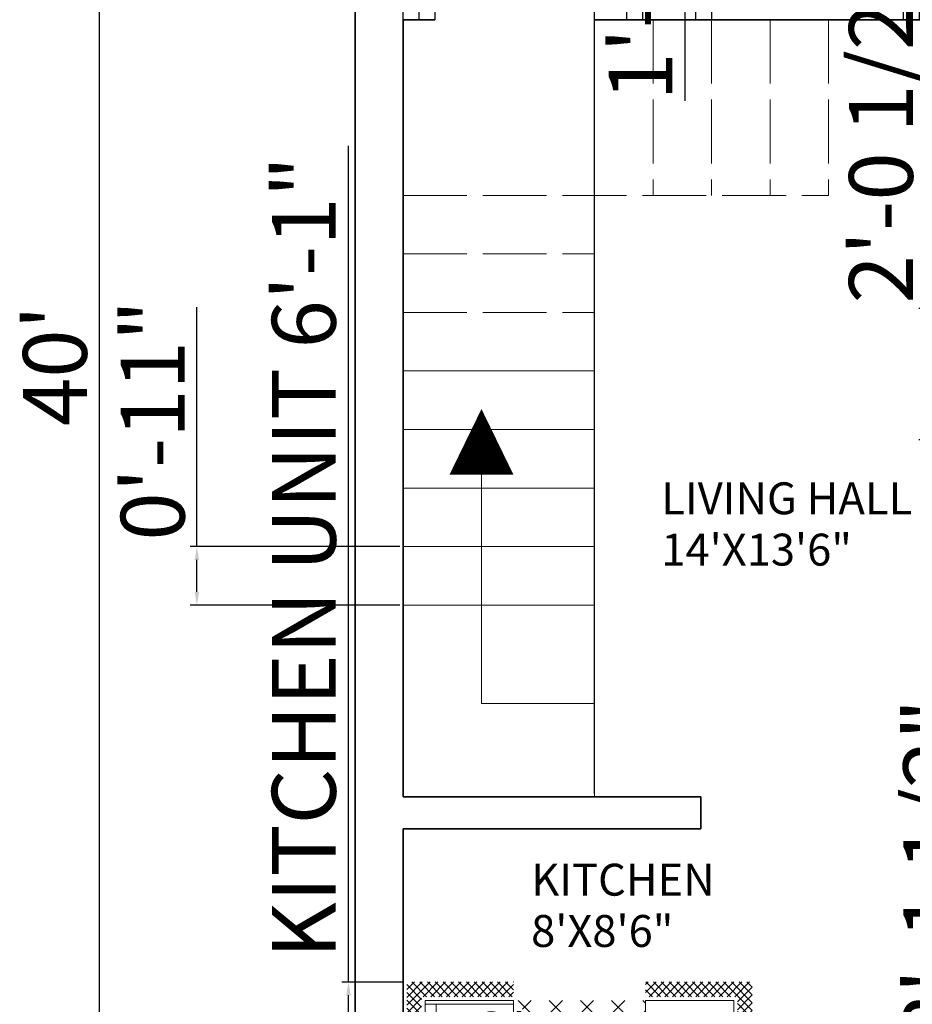
# Model space of a CAD drawing. Units: inches. Extents: x 2353 to 2961, y 642 to 1248.
# Tile 2 of 5: x 2353 to 2520, y 840 to 1025. Entities that reach past the tile are written whole.
import ezdxf

# ---------------------------------------------------------------- set-up
doc = ezdxf.new("R2010")
doc.units = ezdxf.units.IN
doc.linetypes.add('ACAD_ISO02W100', pattern=[15, 12, -3])
for name, color, linetype, lineweight in [('A-ANNO-DIMS', 2, 'Continuous', 18), ('A-AREA-IDEN', 7, 'Continuous', 18), ('A-DOOR', 4, 'Continuous', 25), ('A-FLOR-FIXT', 9, 'Continuous', 18), ('A-FLOR-STRS', 7, 'Continuous', 18), ('A-FLOR-STRS-OVHD', 7, 'ACAD_ISO02W100', 18), ('A-WALL', 7, 'Continuous', 35)]:
    doc.layers.add(name, color=color, linetype=linetype, lineweight=lineweight)
doc.styles.get("Standard").update_dxf_attribs({"font": 'arial.ttf'})
doc.dimstyles.new('ISO-25', dxfattribs={"dimtxt": 12, "dimasz": 2.5, "dimexe": 1.25, "dimexo": 0.625, "dimtad": 1, "dimdec": 1, "dimlunit": 3, "dimtxsty": 'Standard', "dimcen": 2.5, "dimadec": 0, "dimazin": 0, "dimtfac": 1, "dimtdec": 1, "dimtmove": 0, "dimatfit": 3, "dimfxl": 1, "dimarcsym": 0})

# ---------------------------------------------------------------- blocks, each defined once
blk = doc.blocks.new('Kitchen Layout - 7 x 8 ft')
for p, q in [((-5, 81.32), (2.68, 89)), ((-5, 83.44), (0.56, 89)), ((-5, 85.56), (-1.56, 89)), ((-5, 87.68), (-3.68, 89)), ((-1, 84.97), (-5, 88.97)), ((1.09, 85), (-2.91, 89)), ((3.21, 85), (-0.79, 89)), ((0.81, 85), (4.81, 89)), ((5.34, 85), (1.34, 89)), ((2.93, 85), (6.93, 89)), ((7.46, 85), (3.46, 89)), ((5.05, 85), (9.05, 89)), ((9.58, 85), (5.58, 89)), ((7.17, 85), (11.17, 89)), ((11.7, 85), (7.7, 89)), ((9.29, 85), (13.29, 89)), ((13.82, 85), (9.82, 89)), ((11.41, 85), (15.41, 89)), ((15.94, 85), (11.94, 89)), ((13.53, 85), (17.53, 89)), ((18.06, 85), (14.06, 89)), ((15.65, 85), (19.65, 89)), ((20.18, 85), (16.18, 89)), ((17.78, 85), (21.78, 89)), ((22.31, 85), (18.31, 89)), ((19.9, 85), (23.9, 89)), ((24.43, 85), (20.43, 89)), ((22.02, 85), (26.02, 89)), ((26.55, 85), (22.55, 89)), ((24.14, 85), (28.14, 89)), ((28.67, 85), (24.67, 89)), ((26.26, 85), (30.26, 89)), ((30.79, 85), (26.79, 89)), ((28.38, 85), (32.38, 89)), ((32.91, 85), (28.91, 89)), ((30.5, 85), (34.5, 89)), ((35.03, 85), (31.03, 89)), ((32.63, 85), (36.63, 89)), ((37.16, 85), (33.16, 89)), ((34.75, 85), (38.75, 89)), ((39.28, 85), (35.28, 89)), ((36.87, 85), (40.87, 89)), ((41.4, 85), (37.4, 89)), ((38.99, 85), (42.99, 89)), ((43.52, 85), (39.52, 89)), ((41.11, 85), (45.11, 89)), ((45.64, 85), (41.64, 89)), ((43.23, 85), (47.23, 89)), ((47.76, 85), (43.76, 89)), ((45.35, 85), (49.35, 89)), ((49.88, 85), (45.88, 89)), ((47.47, 85), (51.47, 89)), ((52, 85), (48, 89)), ((49.6, 85), (53.6, 89)), ((54.13, 85), (50.13, 89)), ((51.72, 85), (55.72, 89)), ((56.25, 85), (52.25, 89)), ((53.84, 85), (57.84, 89)), ((58.37, 85), (54.37, 89)), ((55.96, 85), (59.96, 89)), ((60.49, 85), (56.49, 89)), ((58.08, 85), (62.08, 89)), ((62.61, 85), (58.61, 89)), ((60.2, 85), (64.2, 89)), ((64.73, 85), (60.73, 89)), ((62.32, 85), (66.32, 89)), ((66.85, 85), (62.85, 89)), ((64.45, 85), (68.45, 89)), ((68.97, 85), (64.97, 89)), ((66.57, 85), (70.57, 89)), ((71.1, 85), (67.1, 89)), ((68.69, 85), (72.69, 89)), ((73.22, 85), (69.22, 89)), ((70.81, 85), (74.81, 89)), ((75.34, 85), (71.34, 89)), ((72.93, 85), (76.93, 89)), ((77.46, 85), (73.46, 89)), ((75.05, 85), (79.05, 89)), ((79.58, 85), (75.58, 89)), ((77.17, 85), (81.17, 89)), ((81.7, 85), (77.7, 89)), ((79.29, 85), (83.29, 89)), ((83.82, 85), (79.82, 89)), ((81.42, 85), (85.42, 89)), ((85.95, 85), (81.95, 89)), ((83.54, 85), (87.54, 89)), ((88.07, 85), (84.07, 89)), ((85.66, 85), (89.66, 89)), ((90.19, 85), (86.19, 89)), ((87.78, 85), (91.78, 89)), ((92.31, 85), (88.31, 89)), ((89.9, 85), (93.9, 89)), ((94.43, 85), (90.43, 89)), ((92.02, 85), (96.02, 89)), ((96.55, 85), (92.55, 89)), ((94.14, 85), (98.14, 89)), ((101, 82.67), (94.67, 89)), ((96.27, 85), (100.27, 89)), ((101, 84.79), (96.79, 89)), ((101, 86.92), (98.92, 89)), ((-1, 82.85), (-5, 86.85)), ((97, 83.61), (101, 87.61)), ((-1, 80.73), (-5, 84.73)), ((-5, 79.19), (-1, 83.19)), ((34, 84), (96, 84)), ((34, 60), (34, 84)), ((96, 84), (96, 60)), ((97, 81.49), (101, 85.49)), ((101, 80.55), (97, 84.55)), ((97, 79.37), (101, 83.37)), ((-1, 78.61), (-5, 82.61)), ((-5, 77.07), (-1, 81.07)), ((-1, 76.49), (-5, 80.49)), ((74, 81), (95, 81)), ((101, 78.43), (97, 82.43)), ((97, 77.25), (101, 81.25)), ((-5, 74.95), (-1, 78.95)), ((-1, 74.36), (-5, 78.36)), ((101, 76.31), (97, 80.31)), ((97, 75.13), (101, 79.13)), ((101, 74.19), (97, 78.19)), ((-5, 72.83), (-1, 76.83)), ((-1, 72.24), (-5, 76.24)), ((97, 73.01), (101, 77.01)), ((101, 72.07), (97, 76.07)), ((-5, 70.71), (-1, 74.71)), ((-1, 70.12), (-5, 74.12)), ((-5, 68.59), (-1, 72.59)), ((97, 70.89), (101, 74.89)), ((101, 69.95), (97, 73.95)), ((97, 68.76), (101, 72.76)), ((-1, 68), (-5, 72)), ((-5, 66.47), (-1, 70.47)), ((-1, 65.88), (-5, 69.88)), ((101, 67.82), (97, 71.82)), ((97, 66.64), (101, 70.64)), ((101, 65.7), (97, 69.7)), ((-5, 64.35), (-1, 68.35)), ((-1, 63.76), (-5, 67.76)), ((97, 64.52), (101, 68.52)), ((101, 63.58), (97, 67.58)), ((-5, 62.22), (-1, 66.22)), ((-1, 61.64), (-5, 65.64)), ((97, 62.4), (101, 66.4)), ((101, 61.46), (97, 65.46)), ((-5, 60.1), (-1, 64.1)), ((-1, 59.52), (-5, 63.52)), ((-5, 57.98), (-1, 61.98)), ((97, 60.28), (101, 64.28)), ((100.34, 60), (97, 63.34)), ((98.84, 60), (101, 62.16)), ((-1, 57.39), (-5, 61.39)), ((-1.73, 56), (-5, 59.27)), ((-4.86, 56), (-1, 59.86)), ((10.4, 24), (45.9, 59.5)), ((18.88, 24), (54.38, 59.5)), ((27.37, 24), (62.87, 59.5)), ((33.03, 55.11), (37.41, 59.5)), ((96, 60), (34, 60)), ((35.85, 24), (71.35, 59.5)), ((76.2, 24), (40.7, 59.5)), ((84.68, 24), (49.18, 59.5)), ((93.17, 24), (57.67, 59.5)), ((96, 29.65), (66.15, 59.5)), ((80, 60), (80, 59)), ((82, 59), (82, 60)), ((87, 59), (87, 60)), ((89, 60), (89, 59)), ((98.22, 60), (97, 61.22)), ((100.96, 60), (101, 60.04)), ((-3.85, 56), (-5, 57.15)), ((-2.74, 56), (-1, 57.74)), ((0, 57), (33, 57)), ((67.71, 24), (33.68, 58.04)), ((44.34, 24), (77.84, 57.5)), ((52.82, 24), (86.32, 57.5)), ((61.31, 24), (96, 58.69)), ((96, 38.14), (76.64, 57.5)), ((96, 46.63), (85.13, 57.5)), ((96, 55.11), (93.57, 57.54)), ((0, 30.57), (24.43, 55)), ((0, 39.06), (15.94, 55)), ((0, 47.54), (7.46, 55)), ((1.91, 24), (32.91, 55)), ((33.77, 24), (2.77, 55)), ((42.26, 24), (11.26, 55)), ((50.74, 24), (19.74, 55)), ((59.23, 24), (28.23, 55)), ((31, 55), (31, 56)), ((32, 55), (31, 55)), ((32, 56), (32, 55)), ((25.29, 24), (0, 49.29)), ((69.79, 24), (96, 50.21)), ((16.8, 24), (0, 40.8)), ((78.28, 24), (96, 41.72)), ((8.32, 24), (0, 32.32)), ((86.76, 24), (96, 33.24)), ((95.25, 24), (96, 24.75)), ((-5, 21.92), (-2.92, 24)), ((-5, 19.8), (-1, 23.8)), ((-1, 19.21), (-5, 23.21)), ((-5, 17.68), (-1, 21.68)), ((-1, 21.33), (-3.67, 24)), ((-1, 23.45), (-1.55, 24)), ((0, 24), (96, 24)), ((0, 0), (0, 24)), ((96, 24), (96, 0)), ((97, 22.1), (98.9, 24)), ((97, 19.97), (101, 23.97)), ((101, 19.03), (97, 23.03)), ((97, 17.85), (101, 21.85)), ((101, 21.16), (98.16, 24)), ((101, 23.28), (100.28, 24)), ((-1, 17.09), (-5, 21.09)), ((-5, 15.55), (-1, 19.55)), ((-1, 14.97), (-5, 18.97)), ((101, 16.91), (97, 20.91)), ((97, 15.73), (101, 19.73)), ((101, 14.79), (97, 18.79)), ((-5, 13.43), (-1, 17.43)), ((-1, 12.85), (-5, 16.85)), ((47.25, 6.5), (47.25, 18.5)), ((48.75, 18.5), (48.75, 6.5)), ((97, 13.61), (101, 17.61)), ((101, 12.67), (97, 16.67)), ((-5, 11.31), (-1, 15.31)), ((-1, 10.73), (-5, 14.73)), ((97, 11.49), (101, 15.49)), ((101, 10.55), (97, 14.55)), ((-5, 9.19), (-1, 13.19)), ((-1, 8.6), (-5, 12.6)), ((-5, 7.07), (-1, 11.07)), ((97, 9.37), (101, 13.37)), ((101, 8.43), (97, 12.43)), ((97, 7.25), (101, 11.25)), ((-1, 6.48), (-5, 10.48)), ((-5, 4.95), (-1, 8.95)), ((-1, 4.36), (-5, 8.36)), ((101, 6.31), (97, 10.31)), ((97, 5.12), (101, 9.12)), ((101, 4.18), (97, 8.18)), ((-5, 2.83), (-1, 6.83)), ((-1, 2.24), (-5, 6.24)), ((97, 3), (101, 7)), ((101, 2.06), (97, 6.06)), ((-5, 0.71), (-1, 4.71)), ((-1, 0.12), (-5, 4.12)), ((64, 4), (32, 4)), ((93.24, -5), (101, 2.76)), ((97, 0.88), (101, 4.88)), ((101, -0.06), (97, 3.94)), ((-5, -1.42), (-1, 2.58)), ((2, -5), (-5, 2)), ((-5, -3.54), (-1, 0.46)), ((96, 0), (0, 0)), ((95.36, -5), (101, 0.64)), ((101, -2.18), (97, 1.82)), ((-0.12, -5), (-5, -0.12)), ((-2.25, -5), (-5, -2.25)), ((-4.34, -5), (-0.34, -1)), ((-2.22, -5), (1.78, -1)), ((-0.1, -5), (3.9, -1)), ((4.12, -5), (0.12, -1)), ((2.02, -5), (6.02, -1)), ((6.24, -5), (2.24, -1)), ((4.14, -5), (8.14, -1)), ((8.36, -5), (4.36, -1)), ((6.27, -5), (10.27, -1)), ((10.48, -5), (6.48, -1)), ((8.39, -5), (12.39, -1)), ((12.6, -5), (8.6, -1)), ((10.51, -5), (14.51, -1)), ((14.73, -5), (10.73, -1)), ((12.63, -5), (16.63, -1)), ((16.85, -5), (12.85, -1)), ((14.75, -5), (18.75, -1)), ((18.97, -5), (14.97, -1)), ((16.87, -5), (20.87, -1)), ((21.09, -5), (17.09, -1)), ((18.99, -5), (22.99, -1)), ((23.21, -5), (19.21, -1)), ((21.11, -5), (25.11, -1)), ((25.33, -5), (21.33, -1)), ((23.24, -5), (27.24, -1)), ((27.45, -5), (23.45, -1)), ((25.36, -5), (29.36, -1)), ((29.57, -5), (25.57, -1)), ((27.48, -5), (30, -2.48)), ((30, -3.3), (27.7, -1)), ((30, -1.18), (29.82, -1)), ((66, -2.54), (67.54, -1)), ((66, -4.66), (69.66, -1)), ((69.88, -5), (66, -1.12)), ((67.78, -5), (71.78, -1)), ((72, -5), (68, -1)), ((69.9, -5), (73.9, -1)), ((74.12, -5), (70.12, -1)), ((72.03, -5), (76.03, -1)), ((76.24, -5), (72.24, -1)), ((74.15, -5), (78.15, -1)), ((78.36, -5), (74.36, -1)), ((76.27, -5), (80.27, -1)), ((80.49, -5), (76.49, -1)), ((78.39, -5), (82.39, -1)), ((82.61, -5), (78.61, -1)), ((80.51, -5), (84.51, -1)), ((84.73, -5), (80.73, -1)), ((82.63, -5), (86.63, -1)), ((86.85, -5), (82.85, -1)), ((84.75, -5), (88.75, -1)), ((88.97, -5), (84.97, -1)), ((86.88, -5), (90.88, -1)), ((91.09, -5), (87.09, -1)), ((89, -5), (93, -1)), ((93.21, -5), (89.21, -1)), ((91.12, -5), (95.12, -1)), ((95.34, -5), (91.34, -1)), ((97.46, -5), (93.46, -1)), ((99.58, -5), (95.58, -1)), ((101, -4.3), (97, -0.3)), ((97.48, -5), (101, -1.48)), ((-4.37, -5), (-5, -4.37)), ((29.6, -5), (30, -4.6)), ((67.76, -5), (66, -3.24)), ((99.6, -5), (101, -3.6))]:
    blk.add_line(p, q)
for points in [[(0, 56), (0, 84), (33, 84), (33, 56)], [(74, 60), (74, 84), (95, 84), (95, 60)], [(76, 58), (76, 59), (93, 59), (93, 58)]]:
    blk.add_lwpolyline(points, close=True)
for points in [[(32, 1.5), (32, 19.5)], [(33.5, 21), (62.5, 21)], [(34.5, 19.5), (46.25, 19.5)], [(49.75, 19.5), (61.5, 19.5)], [(64, 19.5), (64, 1.5)], [(33.5, 6.5), (33.5, 18.5)], [(62.5, 18.5), (62.5, 6.5)], [(46.25, 5.5), (34.5, 5.5)], [(61.5, 5.5), (49.75, 5.5)], [(62.5, 0), (33.5, 0)]]:
    blk.add_lwpolyline(points)
for centre, radius in [((80, 75), 4), ((80, 75), 3), ((89, 75), 3), ((80, 75), 2), ((80, 75), 1), ((89, 75), 2), ((89, 75), 1), ((89, 66), 4), ((80, 66), 3), ((80, 66), 2), ((80, 66), 1), ((89, 66), 3), ((89, 66), 2), ((89, 66), 1), ((40.5, 12.5), 1), ((55.5, 12.5), 1), ((40.5, 12.5), 0.5), ((55.5, 12.5), 0.5)]:
    blk.add_circle(centre, radius)
for centre, radius, start, end in [((33.5, 19.5), 1.5, 90, 180), ((34.5, 18.5), 1, 90, 180), ((46.25, 18.5), 1, 0, 90), ((49.75, 18.5), 1, 90, 180), ((61.5, 18.5), 1, 0, 90), ((62.5, 19.5), 1.5, 0, 90), ((34.5, 6.5), 1, 180, 270), ((46.25, 6.5), 1, 270, 0), ((49.75, 6.5), 1, 180, 270), ((61.5, 6.5), 1, 270, 0), ((33.5, 1.5), 1.5, 180, 270), ((62.5, 1.5), 1.5, 270, 0)]:
    blk.add_arc(centre, radius, start, end)
blk = doc.blocks.new('*D8')
at = {"layer": 'A-ANNO-DIMS', "color": 0, "lineweight": -2, "transparency": 16777216}
for p, q in [((2415.1, 1200.48), (2366.34, 1200.48)), ((2367.59, 1197.98), (2367.59, 722.98)), ((2415.1, 720.48), (2366.34, 720.48))]:
    blk.add_line(p, q, dxfattribs=at)
at = {"layer": 'A-ANNO-DIMS', "color": 0, "transparency": 16777216}
for points in [[(2367.17, 1197.98), (2368.01, 1197.98), (2367.59, 1200.48)], [(2367.17, 722.98), (2368.01, 722.98), (2367.59, 720.48)]]:
    blk.add_solid(points, dxfattribs=at)
at = {"layer": 'Defpoints', "color": 0, "transparency": 16777216}
for p in [(2415.72, 1200.48), (2367.59, 720.48), (2415.72, 720.48)]:
    blk.add_point(p, dxfattribs=at)
at = {"layer": 'A-ANNO-DIMS', "color": 0, "transparency": 16777216, "insert": (2360.84, 960.48), "char_height": 12, "attachment_point": 5, "rotation": 90}
blk.add_mtext("40'", dxfattribs=at)
blk = doc.blocks.new('DOOR-SINGLE-36IN')
for p, q in [((0, 6), (0, 0)), ((3, 6), (3, 0)), ((39, 6), (39, 0)), ((42, 6), (42, 0))]:
    blk.add_line(p, q)
blk.add_lwpolyline([(3, 6), (6, 6), (6, 42), (3, 42)], close=True)
blk.add_arc((4.5, 7.5), 34.53, 357.5104, 92.4896)
blk = doc.blocks.new('*D20')
at = {"layer": 'A-ANNO-DIMS', "color": 0, "lineweight": -2, "transparency": 16777216}
for p, q in [((2473.35, 1106.99), (2478.93, 1106.99)), ((2477.68, 1104.49), (2477.68, 1088.49)), ((2473.35, 1085.99), (2478.93, 1085.99)), ((2477.68, 1085.99), (2477.68, 1010.22))]:
    blk.add_line(p, q, dxfattribs=at)
at = {"layer": 'A-ANNO-DIMS', "color": 0, "transparency": 16777216}
for points in [[(2477.26, 1104.49), (2478.1, 1104.49), (2477.68, 1106.99)], [(2477.26, 1088.49), (2478.1, 1088.49), (2477.68, 1085.99)]]:
    blk.add_solid(points, dxfattribs=at)
at = {"layer": 'Defpoints', "color": 0, "transparency": 16777216}
for p in [(2472.72, 1106.99), (2472.72, 1085.99), (2477.68, 1085.99)]:
    blk.add_point(p, dxfattribs=at)
at = {"layer": 'A-ANNO-DIMS', "color": 0, "transparency": 16777216, "insert": (2470.93, 1046.86), "char_height": 12, "attachment_point": 5, "rotation": 90}
blk.add_mtext('1\'-9" TYP.', dxfattribs=at)
blk = doc.blocks.new('*D22')
at = {"layer": 'A-ANNO-DIMS', "color": 0, "lineweight": -2, "transparency": 16777216}
for p, q in [((2522.95, 971.22), (2522.95, 1035.04)), ((2528.38, 971.22), (2521.7, 971.22)), ((2522.95, 949.04), (2522.95, 968.72)), ((2528.38, 946.54), (2521.7, 946.54))]:
    blk.add_line(p, q, dxfattribs=at)
at = {"layer": 'A-ANNO-DIMS', "color": 0, "transparency": 16777216}
for points in [[(2522.54, 968.72), (2523.37, 968.72), (2522.95, 971.22)], [(2522.54, 949.04), (2523.37, 949.04), (2522.95, 946.54)]]:
    blk.add_solid(points, dxfattribs=at)
at = {"layer": 'Defpoints', "color": 0, "transparency": 16777216}
for p in [(2522.95, 971.22), (2529.01, 971.22), (2529.01, 946.54)]:
    blk.add_point(p, dxfattribs=at)
at = {"layer": 'A-ANNO-DIMS', "color": 0, "transparency": 16777216, "insert": (2516.12, 1004.38), "char_height": 12, "attachment_point": 5, "rotation": 90}
blk.add_mtext('2\'-0 1/2"', dxfattribs=at)
blk = doc.blocks.new('*D25')
at = {"layer": 'A-ANNO-DIMS', "color": 0, "lineweight": -2, "transparency": 16777216}
for p, q in [((2538.14, 943.02), (2531.92, 943.02)), ((2533.17, 940.52), (2533.17, 908.21)), ((2538.14, 905.71), (2531.92, 905.71)), ((2533.17, 905.71), (2533.17, 711.83))]:
    blk.add_line(p, q, dxfattribs=at)
at = {"layer": 'A-ANNO-DIMS', "color": 0, "transparency": 16777216}
for points in [[(2532.75, 940.52), (2533.58, 940.52), (2533.17, 943.02)], [(2532.75, 908.21), (2533.58, 908.21), (2533.17, 905.71)]]:
    blk.add_solid(points, dxfattribs=at)
at = {"layer": 'Defpoints', "color": 0, "transparency": 16777216}
for p in [(2538.76, 943.02), (2533.17, 905.71), (2538.76, 905.71)]:
    blk.add_point(p, dxfattribs=at)
at = {"layer": 'A-ANNO-DIMS', "color": 0, "transparency": 16777216, "insert": (2526.33, 807.52), "char_height": 12, "attachment_point": 5, "rotation": 90}
blk.add_mtext('COFFEE TABLE 3\'-1 1/2"', dxfattribs=at)
blk = doc.blocks.new('*D31')
at = {"layer": 'A-ANNO-DIMS', "color": 0, "lineweight": -2, "transparency": 16777216}
for p, q in [((2414.46, 844.67), (2414.46, 1001.8)), ((2424.82, 844.67), (2413.21, 844.67)), ((2414.46, 773.98), (2414.46, 842.17)), ((2424.82, 771.48), (2413.21, 771.48))]:
    blk.add_line(p, q, dxfattribs=at)
at = {"layer": 'A-ANNO-DIMS', "color": 0, "transparency": 16777216}
for points in [[(2414.05, 842.17), (2414.88, 842.17), (2414.46, 844.67)], [(2414.05, 773.98), (2414.88, 773.98), (2414.46, 771.48)]]:
    blk.add_solid(points, dxfattribs=at)
at = {"layer": 'Defpoints', "color": 0, "transparency": 16777216}
for p in [(2414.46, 844.67), (2425.44, 844.67), (2425.44, 771.48)]:
    blk.add_point(p, dxfattribs=at)
at = {"layer": 'A-ANNO-DIMS', "color": 0, "transparency": 16777216, "insert": (2407.63, 924.49), "char_height": 12, "attachment_point": 5, "rotation": 90}
blk.add_mtext('KITCHEN UNIT 6\'-1"', dxfattribs=at)
blk = doc.blocks.new('*D35')
at = {"layer": 'A-ANNO-DIMS', "color": 0, "lineweight": -2, "transparency": 16777216}
for p, q in [((2424.72, 880.11), (2424.72, 1231.48)), ((2460.72, 880.11), (2460.72, 1231.48)), ((2427.22, 1230.23), (2458.22, 1230.23))]:
    blk.add_line(p, q, dxfattribs=at)
at = {"layer": 'A-ANNO-DIMS', "color": 0, "transparency": 16777216}
for points in [[(2427.22, 1230.65), (2427.22, 1229.82), (2424.72, 1230.23)], [(2458.22, 1230.65), (2458.22, 1229.82), (2460.72, 1230.23)]]:
    blk.add_solid(points, dxfattribs=at)
at = {"layer": 'Defpoints', "color": 0, "transparency": 16777216}
for p in [(2460.72, 1230.23), (2424.72, 879.48), (2460.72, 879.48)]:
    blk.add_point(p, dxfattribs=at)
at = {"layer": 'A-ANNO-DIMS', "color": 0, "transparency": 16777216, "insert": (2442.72, 1236.99), "char_height": 12, "attachment_point": 5}
blk.add_mtext('3\'-0"', dxfattribs=at)
blk = doc.blocks.new('*D36')
at = {"layer": 'A-ANNO-DIMS', "color": 0, "lineweight": -2, "transparency": 16777216}
for p, q in [((2385.97, 926.48), (2385.97, 971.46)), ((2424.1, 926.48), (2384.72, 926.48)), ((2385.97, 917.98), (2385.97, 923.98)), ((2424.1, 915.48), (2384.72, 915.48))]:
    blk.add_line(p, q, dxfattribs=at)
at = {"layer": 'A-ANNO-DIMS', "color": 0, "transparency": 16777216}
for points in [[(2385.56, 923.98), (2386.39, 923.98), (2385.97, 926.48)], [(2385.56, 917.98), (2386.39, 917.98), (2385.97, 915.48)]]:
    blk.add_solid(points, dxfattribs=at)
at = {"layer": 'Defpoints', "color": 0, "transparency": 16777216}
for p in [(2385.97, 926.48), (2424.72, 926.48), (2424.72, 915.48)]:
    blk.add_point(p, dxfattribs=at)
at = {"layer": 'A-ANNO-DIMS', "color": 0, "transparency": 16777216, "insert": (2379.22, 950.22), "char_height": 12, "attachment_point": 5, "rotation": 90}
blk.add_mtext('0\'-11"', dxfattribs=at)

msp = doc.modelspace()

# ---------------------------------------------------------------- linework, layer by layer
at = {"layer": 'A-FLOR-STRS'}
for p, q in [((2460.72, 992.48), (2460.72, 879.48)), ((2424.72, 959.48), (2460.72, 959.48)), ((2424.72, 948.48), (2460.72, 948.48)), ((2424.72, 937.48), (2460.72, 937.48)), ((2424.72, 926.48), (2460.72, 926.48)), ((2424.72, 915.48), (2460.72, 915.48))]:
    msp.add_line(p, q, dxfattribs=at)
msp.add_lwpolyline([(2439.47, 940.02, 12, 0, 0), (2439.47, 952.34, 0, 0, 0)], format="xyseb", dxfattribs=at)
msp.add_lwpolyline([(2460.72, 896.98), (2439.47, 896.98), (2439.47, 940.02)], dxfattribs=at)
at = {"layer": 'A-FLOR-STRS-OVHD'}
for p, q in [((2460.72, 992.48), (2460.72, 1025.48)), ((2471.72, 1025.48), (2471.72, 992.48)), ((2482.72, 1025.48), (2482.72, 992.48)), ((2493.72, 1025.48), (2493.72, 992.48)), ((2504.72, 1025.48), (2504.72, 992.48)), ((2424.72, 992.48), (2504.72, 992.48)), ((2424.72, 981.48), (2460.72, 981.48)), ((2424.72, 970.48), (2460.72, 970.48))]:
    msp.add_line(p, q, dxfattribs=at)
at = {"layer": 'A-WALL'}
for p, q in [((2424.72, 1025.48), (2424.72, 879.48)), ((2430.72, 1025.48), (2424.72, 1025.48)), ((2586.72, 1025.48), (2460.72, 1025.48)), ((2424.72, 879.48), (2480.72, 879.48)), ((2480.72, 873.48), (2480.72, 879.48)), ((2424.72, 873.48), (2480.72, 873.48)), ((2424.72, 873.48), (2424.72, 771.48))]:
    msp.add_line(p, q, dxfattribs=at)
msp.add_lwpolyline([(2574.3, 720.48), (2595.72, 720.48), (2595.72, 1200.48), (2415.72, 1200.48), (2415.72, 720.48), (2445.67, 720.48)], dxfattribs=at)

# ---------------------------------------------------------------- block references
at = {"layer": 'A-DOOR', "extrusion": (0, 0, -1), "zscale": -1}
msp.add_blockref('DOOR-SINGLE-36IN', (-2469.72, 1025.48), dxfattribs=at)
at = {"layer": 'A-DOOR'}
msp.add_blockref('DOOR-SINGLE-36IN', (2479.72, 1025.48), dxfattribs=at)
at = {"layer": 'A-FLOR-FIXT', "xscale": 0.690484494816598, "yscale": 0.690484494816598, "zscale": 0.690484494816598, "rotation": 90}
msp.add_blockref('Kitchen Layout - 7 x 8 ft', (2486.89, 774.94), dxfattribs=at)

# ---------------------------------------------------------------- texts
at = {"layer": 'A-AREA-IDEN'}
for s, p in [('LIVING HALL', (2473.27, 932.55)), ('14\'X13\'6"', (2473.27, 922.91)), ('KITCHEN', (2448.8, 860.9)), ('8\'X8\'6"', (2448.8, 851.26))]:
    msp.add_text(s, height=6, dxfattribs=at).set_placement(p)

# ---------------------------------------------------------------- dimensions: what is measured, and where the dimension line sits
at = {"layer": 'A-ANNO-DIMS'}
dim = msp.add_linear_dim(base=(2460.72, 1230.23), p1=(2424.72, 879.48), p2=(2460.72, 879.48), dimstyle='ISO-25', override={"dimdec": 1, "dimlfac": 1, "dimrnd": 0, "dimzin": 1, "dimdsep": 46, "dimlunit": 4, "dimfrac": 2}, dxfattribs=at)
dim.commit()
dim.dimension.update_dxf_attribs({"geometry": '*D35', "text_midpoint": (2442.72, 1236.99)})
for base, p1, p2, override, picture, middle in [((2367.59, 720.48), (2415.72, 1200.48), (2415.72, 720.48), {"dimclrd": 0, "dimclre": 0, "dimclrt": 0}, '*D8', (2360.84, 960.48)), ((2522.95, 971.22), (2529.01, 946.54), (2529.01, 971.22), {"dimdec": 1, "dimlfac": 1, "dimrnd": 0, "dimzin": 1, "dimdsep": 46, "dimlunit": 4, "dimfrac": 2}, '*D22', (2516.12, 1004.38)), ((2385.97, 926.48), (2424.72, 915.48), (2424.72, 926.48), {"dimdec": 1, "dimlfac": 1, "dimrnd": 0, "dimzin": 1, "dimdsep": 46, "dimlunit": 4, "dimfrac": 2}, '*D36', (2379.22, 950.22))]:
    dim = msp.add_linear_dim(base=base, p1=p1, p2=p2, angle=90, dimstyle='ISO-25', override=override, dxfattribs=at)
    dim.commit()
    dim.dimension.update_dxf_attribs({"geometry": picture, "text_midpoint": middle})
for base, p1, p2, angle, text, picture, middle in [((2477.68, 1085.99), (2472.72, 1106.99), (2472.72, 1085.99), 270, '<> TYP.', '*D20', (2470.93, 1046.86)), ((2414.46, 844.67), (2425.44, 771.48), (2425.44, 844.67), 90, 'KITCHEN UNIT <>', '*D31', (2407.63, 924.49)), ((2533.17, 905.71), (2538.76, 943.02), (2538.76, 905.71), 270, 'COFFEE TABLE <>', '*D25', (2526.33, 807.52))]:
    dim = msp.add_linear_dim(base=base, p1=p1, p2=p2, angle=angle, text=text, dimstyle='ISO-25', override={"dimdec": 1, "dimlfac": 1, "dimrnd": 0, "dimzin": 1, "dimdsep": 46, "dimlunit": 4, "dimfrac": 2}, dxfattribs=at)
    dim.commit()
    dim.dimension.update_dxf_attribs({"geometry": picture, "text_midpoint": middle})

doc.saveas('drawing.dxf')
